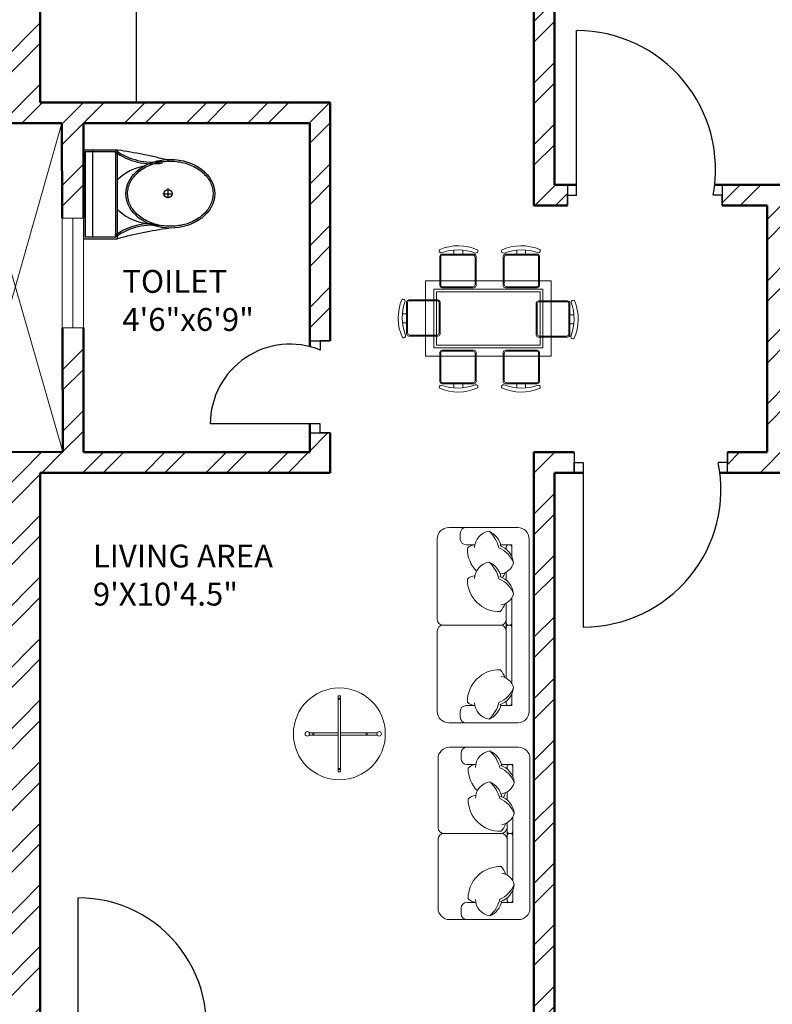
# Model space of a CAD drawing. Units: inches. Extents: x 1980 to 2738, y 1471 to 2568.
# Tile 20 of 22: x 2363 to 2528, y 2112 to 2328. Entities that reach past the tile are written whole.
import ezdxf

# ---------------------------------------------------------------- set-up
doc = ezdxf.new("R2010")
doc.units = ezdxf.units.IN
for name, color, linetype, lineweight in [('A-ANNO-DIMS', 2, 'Continuous', 18), ('A-AREA-IDEN', 7, 'Continuous', 18), ('A-DOOR', 31, 'Continuous', 25), ('A-FLOR-CASE', 8, 'Continuous', 25), ('A-FLOR-FIXT', 8, 'Continuous', 25), ('A-FLOR-OPEN', 8, 'Continuous', 18), ('A-FURN', 8, 'Continuous', 18), ('A-GLAZ', 141, 'Continuous', 18), ('A-WALL', 7, 'Continuous', 50)]:
    doc.layers.add(name, color=color, linetype=linetype, lineweight=lineweight)
doc.layers.add('A-WALL-PATT', color=9, linetype='Continuous', lineweight=13, true_color=0xd19cc7)
doc.styles.get("Standard").update_dxf_attribs({"font": 'arial.ttf'})
doc.dimstyles.get("Standard").update_dxf_attribs({"dimtxt": 0.18, "dimasz": 0.18, "dimexe": 0.18, "dimexo": 0.0625, "dimgap": 0.09, "dimtad": 0, "dimtih": 1, "dimtoh": 1, "dimdec": 4, "dimzin": 0, "dimdsep": 46, "dimtxsty": 'Standard', "dimcen": 0.09, "dimadec": 0, "dimazin": 0, "dimtfac": 1, "dimtdec": 4, "dimtofl": 0, "dimtmove": 0, "dimatfit": 3, "dimfxl": 1, "dimtolj": 1, "dimtzin": 0, "dimarcsym": 0})

# ---------------------------------------------------------------- blocks, each defined once
blk = doc.blocks.new('A$C31115884')
for p, q in [((257.5, 466.4), (257.5, 523.2)), ((283.1, 497.7), (223.4, 497.7)), ((0, 200), (0, 0)), ((520, 200), (0, 200)), ((10, 190), (10, 10)), ((510, 190), (10, 190)), ((510, 10), (510, 190)), ((520, 0), (520, 200)), ((510, 54.5), (0, 54.5)), ((10, 10), (510, 10)), ((0, 0), (520, 0))]:
    blk.add_line(p, q)
blk.add_circle((255.6, 496.4), 23.6)
for centre, radius, start, end in [((2777.7, -204.6), 2807, 165.4549, 171.71327), ((-294.5, 403.3), 364.7, 324.20913, 9.34987), ((-294.5, 403.3), 374.7, 324.20913, 9.34987), ((805.8, 403.3), 364.7, 170.65013, 215.79087), ((3237, 905), 2807, 188.28673, 194.5451), ((139.5, 406.2), 293.5, 315.84364, 2.65635), ((805.8, 403.3), 374.7, 179.20365, 215.79087), ((383.6, 406.2), 293.5, 190.27735, 224.15636)]:
    blk.add_arc(centre, radius, start, end)
blk.add_ellipse((256.2, 509.9), major_axis=(0, -260.7), ratio=0.772727)
blk.add_open_spline([(256.2, 259.2), (263.1, 259.2), (270, 259.7), (287.8, 262.3), (298.7, 265.1), (319.9, 273.1), (330.2, 278.4), (350.1, 291.1), (359.7, 298.7), (377.7, 315.9), (386.2, 325.5), (401.7, 346.6), (408.8, 358.1), (421.3, 382.5), (426.8, 395.5), (435.9, 422.4), (439.5, 436.4), (444.8, 465.1), (446.5, 479.7), (447.9, 509.2), (447.6, 524), (445, 553.3), (442.7, 567.8), (436.3, 596), (432.1, 609.7), (421.9, 636), (416, 648.6), (402.5, 672.1), (395, 683), (378.6, 703), (369.8, 712.1), (351.1, 728), (341.3, 734.8), (320.9, 746.2), (310.4, 750.7), (288.9, 757.3), (278, 759.4), (256, 761), (245, 760.6), (223.1, 757.2), (212.3, 754.3), (191.1, 746.1), (180.8, 740.7), (160.9, 727.8), (151.4, 720.1), (133.5, 702.7), (125.1, 693), (109.6, 671.7), (102.6, 660.2), (90.2, 635.7), (84.9, 622.7), (76, 595.6), (72.4, 581.6), (67.2, 552.9), (65.6, 538.2), (64.4, 508.8), (64.8, 494), (67.5, 464.7), (69.9, 450.2), (76.6, 422), (80.8, 408.3), (91.1, 382.2), (97.2, 369.7), (110.8, 346.3), (118.4, 335.4), (134.8, 315.6), (143.7, 306.7), (162.4, 290.9), (172.3, 284.2), (192.8, 273), (203.3, 268.6), (224.8, 262.2), (235.8, 260.2), (249.9, 259.3), (253, 259.2), (256.2, 259.2)], degree=3, knots=[0, 0, 0, 0, 0.110105, 0.110105, 0.285049, 0.285049, 0.459994, 0.459994, 0.634938, 0.634938, 0.809882, 0.809882, 0.984827, 0.984827, 1.159771, 1.159771, 1.334715, 1.334715, 1.50966, 1.50966, 1.684604, 1.684604, 1.859549, 1.859549, 2.034493, 2.034493, 2.209437, 2.209437, 2.384382, 2.384382, 2.559326, 2.559326, 2.73427, 2.73427, 2.909215, 2.909215, 3.084159, 3.084159, 3.259103, 3.259103, 3.434048, 3.434048, 3.608992, 3.608992, 3.783936, 3.783936, 3.958881, 3.958881, 4.133825, 4.133825, 4.30877, 4.30877, 4.483714, 4.483714, 4.658658, 4.658658, 4.833603, 4.833603, 5.008547, 5.008547, 5.183491, 5.183491, 5.358436, 5.358436, 5.53338, 5.53338, 5.708324, 5.708324, 5.883269, 5.883269, 6.058213, 6.058213, 6.233158, 6.233158, 6.283185, 6.283185, 6.283185, 6.283185])
blk = doc.blocks.new('table r 343')
at = {"color": 0}
for p, q in [((-10, 10), (-10, 262.1)), ((10, 10), (10, 262.1)), ((-330.3, 10), (330.3, 10)), ((-330.3, 10), (-330.3, -10)), ((330.3, 10), (330.3, -10)), ((-330.3, -10), (330.3, -10)), ((-10, -330.3), (-10, -10)), ((10, -330.3), (10, -10))]:
    blk.add_line(p, q, dxfattribs=at)
for centre, radius in [((0, 0), 400), ((0, 278.7), 19.4), ((0, 226.8), 5), ((-306.1, 0), 5), ((306.1, 0), 5), ((0, -238.1), 5), ((0, -346.9), 19.4)]:
    blk.add_circle(centre, radius, dxfattribs=at)
blk = doc.blocks.new('TABLE-DINING-RECT')
for points in [[(0, 16.47), (27.45, 16.47), (27.45, 0), (0, 0)], [(0, 16.47), (27.45, 16.47), (27.45, 0), (0, 0)], [(1.83, 14.64), (25.62, 14.64), (25.62, 1.83), (1.83, 1.83)], [(1.83, 14.64), (25.62, 14.64), (25.62, 1.83), (1.83, 1.83)], [(2.38, 14.09), (25.07, 14.09), (25.07, 2.38), (2.38, 2.38)], [(2.38, 14.09), (25.07, 14.09), (25.07, 2.38), (2.38, 2.38)]]:
    blk.add_lwpolyline(points, close=True)
blk = doc.blocks.new('CHAIR-DINING')
for points in [[(0.45, 7.65, -0.175809), (7.92, 7.6, 0.578392), (8.49, 8.22, 0.214524), (0.05, 8.33, 0.552014), (0.45, 7.65, -0.065079)], [(0.45, 7.65, -0.175809), (7.92, 7.6, 0.578392), (8.49, 8.22, 0.214524), (0.05, 8.33, 0.552014), (0.45, 7.65, -0.065079)], [(7.61, 7.35), (0.67, 7.35, 0.414214), (0.18, 6.87), (0.18, 0.49, 0.414214), (0.67, 0), (7.61, 0, 0.414214), (8.09, 0.49), (8.09, 6.87, 0.414214), (7.61, 7.35)], [(7.61, 7.35), (0.67, 7.35, 0.414214), (0.18, 6.87), (0.18, 0.49, 0.414214), (0.67, 0), (7.61, 0, 0.414214), (8.09, 0.49), (8.09, 6.87, 0.414214), (7.61, 7.35)], [(5.17, 7.35), (5.17, 8.23, -0.064759)], [(5.17, 7.35), (5.17, 8.23, -0.064759)]]:
    blk.add_lwpolyline(points, format="xyb")
blk.add_lwpolyline([(0.67, 7.13), (7.39, 7.13, -0.414214), (7.87, 6.65), (7.87, 0.7, -0.414214), (7.39, 0.22), (0.67, 0.22, -0.512069), (0.4, 0.7), (0.4, 6.65, -0.512069)], format="xyb", close=True)
blk.add_lwpolyline([(0.67, 7.13), (7.39, 7.13, -0.414214), (7.87, 6.65), (7.87, 0.7, -0.414214), (7.39, 0.22), (0.67, 0.22, -0.512069), (0.4, 0.7), (0.4, 6.65, -0.512069)], format="xyb", close=True)
blk.add_lwpolyline([(3.23, 8.25), (3.23, 7.35)])
blk.add_lwpolyline([(3.23, 8.25), (3.23, 7.35)])
blk = doc.blocks.new('SHAFT-OPENING-MARK')
for p, q in [((20.51, 72), (0, 0)), ((0, 72), (20.71, 0.06))]:
    blk.add_line(p, q)
blk = doc.blocks.new('*D35')
at = {"layer": 'A-ANNO-DIMS', "color": 0, "lineweight": -2, "transparency": 16777216}
for p, q in [((2081.08, 2291.77), (2081.08, 2507.54)), ((2081.26, 2507.36), (2362.79, 2507.36)), ((2644.9, 2507.36), (2363.37, 2507.36)), ((2645.08, 2291.77), (2645.08, 2507.54))]:
    blk.add_line(p, q, dxfattribs=at)
at = {"layer": 'A-ANNO-DIMS', "color": 0, "transparency": 16777216}
for points in [[(2081.26, 2507.39), (2081.26, 2507.33), (2081.08, 2507.36)], [(2644.9, 2507.39), (2644.9, 2507.33), (2645.08, 2507.36)]]:
    blk.add_solid(points, dxfattribs=at)
at = {"layer": 'Defpoints', "color": 0, "transparency": 16777216}
for p in [(2645.08, 2507.36), (2081.08, 2291.71), (2645.08, 2291.71)]:
    blk.add_point(p, dxfattribs=at)
at = {"layer": 'A-ANNO-DIMS', "color": 0, "transparency": 16777216, "insert": (2363.08, 2507.36), "char_height": 0.18, "attachment_point": 5}
blk.add_mtext('\\A1;564', dxfattribs=at)

msp = doc.modelspace()

# ---------------------------------------------------------------- hatches: boundary and pattern name
at = {"layer": 'A-WALL-PATT'}
h = msp.add_hatch(dxfattribs=at)
h.set_pattern_fill('ANSI32', color=256)
h.paths.add_polyline_path([(2257.5661, 2416.2064), (2257.5661, 2420.7064), (2250.5833, 2420.7064), (2250.5833, 2462.7064), (2246.0833, 2462.7064), (2246.0833, 2420.7064), (2237.0791, 2420.7064), (2237.0791, 2411.7064), (2246.0833, 2411.7064), (2246.0833, 2291.7064), (2242.6109, 2291.7064), (2242.6109, 2287.2064), (2246.0833, 2287.2064), (2250.5833, 2287.2064), (2250.5833, 2291.7064), (2250.5833, 2411.7064), (2257.5661, 2411.7064)])
h.paths.add_polyline_path([(2387.0396, 2416.2064), (2387.0396, 2420.7064), (2367.5833, 2420.7064), (2367.5833, 2462.7064), (2358.5833, 2462.7064), (2358.5833, 2420.7064), (2329.3087, 2420.7064), (2329.3087, 2411.7064), (2358.5833, 2411.7064), (2358.5833, 2321.7275), (2358.5833, 2309.7064), (2347.3089, 2309.7064), (2293.3089, 2309.7064), (2293.3089, 2259.0771), (2297.8089, 2259.0771), (2297.8089, 2305.2064), (2347.3089, 2305.2064), (2347.3089, 2284.7412), (2351.8089, 2284.7412), (2351.8089, 2305.2064), (2372.3188, 2305.2064), (2372.3761, 2284.3899), (2377.0295, 2284.3899), (2377.0295, 2299.3058), (2377.0295, 2305.2064), (2426.5295, 2305.2064), (2426.5295, 2257.5573), (2431.0295, 2257.5573), (2431.0295, 2309.7064), (2377.0295, 2309.7064), (2367.5833, 2309.7064), (2367.5833, 2321.7275), (2367.5833, 2411.7064), (2387.0396, 2411.7064)])
h.paths.add_polyline_path([(2448.5267, 2416.2064), (2448.5267, 2420.7064), (2423.0396, 2420.7064), (2423.0396, 2411.7064), (2448.5267, 2411.7064)])
h.paths.add_polyline_path([(2130.9128, 2416.2064), (2130.9128, 2420.7064), (2105.0833, 2420.7064), (2105.0833, 2386.6942), (2114.0833, 2386.6942), (2114.0833, 2411.7064), (2130.9128, 2411.7064)])
h.paths.add_polyline_path([(2212.9478, 2420.7064), (2190.9128, 2420.7064), (2190.9128, 2411.7064), (2212.9478, 2411.7064), (2212.9478, 2416.2064)])
h.paths.add_polyline_path([(2114.0833, 2326.6942), (2105.0833, 2326.6942), (2105.0833, 2291.7064), (2081.0833, 2291.7064), (2081.0833, 2287.2064), (2105.0833, 2287.2064), (2105.0833, 2276.1935), (2114.0833, 2276.1935), (2114.0833, 2287.2064), (2166.3825, 2287.2064), (2166.3825, 2289.4564), (2166.3825, 2291.7064), (2114.0833, 2291.7064)])
h.paths.add_polyline_path([(2114.0833, 2252.1935), (2105.0833, 2252.1935), (2105.0833, 2233.2064), (2081.0833, 2233.2064), (2081.0833, 2228.7064), (2105.0833, 2228.7064), (2105.0833, 2213.4478), (2114.0833, 2213.4478), (2114.0833, 2228.7064), (2195.0833, 2228.7064), (2199.5833, 2228.7064), (2208.4455, 2228.7064), (2208.4455, 2230.9564), (2208.4455, 2233.2064), (2199.5833, 2233.2064), (2199.5833, 2287.2064), (2206.8904, 2287.2064), (2206.8904, 2289.4564), (2206.8904, 2291.7064), (2189.446, 2291.7064), (2189.446, 2289.4564), (2189.446, 2287.2064), (2195.0833, 2287.2064), (2195.0833, 2233.2064), (2114.0833, 2233.2064)])
h.paths.add_polyline_path([(2114.0833, 2153.4478), (2109.5833, 2153.4478), (2105.0833, 2153.4478), (2105.0833, 2135.2374), (2114.0833, 2135.2374)], flags=17)
h.paths.add_polyline_path([(2135.9619, 2095.4081), (2140.1805, 2095.4081), (2140.1805, 2104.2064), (2114.0833, 2104.2064), (2114.0833, 2110.3997), (2109.5833, 2110.3997), (2105.0833, 2110.3997), (2105.0833, 2104.2064), (2081.0833, 2104.2064), (2081.0833, 2099.7064), (2105.0833, 2099.7064), (2127.5416, 2099.8532), (2127.5416, 2056.9393), (2136.2133, 2056.9393)], flags=17)
h.paths.add_polyline_path([(2255.4895, 2104.2064), (2250.5833, 2104.2064), (2250.5833, 2233.2064), (2246.0833, 2233.2064), (2242.4941, 2233.2064), (2242.4941, 2228.7064), (2246.0833, 2228.7064), (2246.0833, 2104.2064), (2163.6825, 2104.2064), (2163.6825, 2099.8072), (2163.6825, 2095.4081), (2191.4325, 2095.4081), (2191.4325, 2011.2064), (2186.0833, 2011.2064), (2136.5143, 2010.8824), (2136.3702, 2032.9403), (2131.9559, 2032.9115), (2127.5416, 2032.8826), (2127.5416, 2006.7064), (2105.0833, 2006.7064), (2081.0833, 2006.7064), (2081.0833, 2002.2064), (2105.0833, 2002.2064), (2105.0833, 1995.9329), (2114.0833, 1995.9329), (2114.0833, 2002.2064), (2246.0833, 2002.2064), (2246.0833, 1877.7064), (2242.1358, 1877.7064), (2242.1358, 1873.2064), (2250.5833, 1873.2064), (2250.5833, 2002.2064), (2255.3335, 2002.2064), (2255.3335, 2011.2064), (2195.9325, 2011.2064), (2195.9325, 2095.2064), (2255.4895, 2095.2064), (2255.4895, 2099.5471)])
h.paths.add_polyline_path([(2199.5833, 1873.2064), (2209.827, 1873.2064), (2209.827, 1875.4564), (2209.827, 1877.7064), (2114.0833, 1877.7064), (2114.0833, 1890.0968), (2105.0833, 1890.0968), (2105.0833, 1877.7064), (2081.0833, 1877.7064), (2081.0833, 1873.2064), (2105.0833, 1873.2064), (2105.0833, 1857.7279), (2114.0833, 1857.7279), (2114.0833, 1873.2064), (2195.0833, 1873.2064), (2195.0833, 1819.2064), (2190.298, 1819.2064), (2190.298, 1814.7064), (2209.8976, 1814.7064), (2209.8976, 1816.9564), (2209.8976, 1819.2064), (2199.5833, 1819.2064)])
h.paths.add_polyline_path([(2114.0833, 1814.7064), (2166.2538, 1814.7064), (2166.2538, 1816.9564), (2166.2538, 1819.2064), (2114.0833, 1819.2064), (2114.0833, 1833.7279), (2109.5833, 1833.7279), (2105.0833, 1833.7279), (2105.0833, 1819.2064), (2081.0833, 1819.2064), (2081.0833, 1814.7064), (2105.0833, 1814.7064), (2105.0833, 1782.5516), (2114.0833, 1782.5516)])
h.paths.add_polyline_path([(2114.0833, 1722.5516), (2109.5833, 1722.5516), (2105.0833, 1722.5516), (2105.0833, 1685.7064), (2124.5104, 1685.7064), (2124.5104, 1690.2064), (2124.5104, 1694.7064), (2114.0833, 1694.7064)])
h.paths.add_polyline_path([(2218.8787, 1694.7064), (2184.5104, 1694.7064), (2184.5104, 1685.7064), (2218.8787, 1685.7064), (2218.8787, 1690.2064)])
h.paths.add_polyline_path([(2250.5833, 1819.2064), (2242.6431, 1819.2064), (2242.6431, 1816.9564), (2242.6431, 1814.7064), (2246.0833, 1814.7064), (2246.0833, 1694.7064), (2240.4035, 1694.7064), (2240.4035, 1690.2064), (2240.4035, 1685.7064), (2246.0833, 1685.7064), (2246.0833, 1643.7064), (2250.5833, 1643.7064), (2250.5833, 1685.7064), (2255.9859, 1685.7064), (2255.9859, 1690.2064), (2255.9859, 1694.7064), (2250.5833, 1694.7064)])
h.paths.add_polyline_path([(2297.4764, 1694.7064), (2279.3934, 1694.7064), (2279.3934, 1690.2064), (2279.3934, 1685.7064), (2297.4764, 1685.7064), (2297.4764, 1690.2064)])
h.paths.add_polyline_path([(2377.1596, 1694.7064), (2367.5833, 1694.7064), (2367.5833, 1787.7064), (2431.0295, 1787.7064), (2431.0295, 1792.2064), (2431.0295, 1849.4149), (2428.7795, 1849.4149), (2426.5295, 1849.4149), (2426.5295, 1792.2064), (2421.5833, 1792.2064), (2367.5833, 1792.2064), (2297.8089, 1792.2064), (2297.8089, 1850.2946), (2295.5589, 1850.2946), (2293.3089, 1850.2946), (2293.3089, 1792.2064), (2293.3089, 1787.7064), (2297.8089, 1787.7064), (2358.5833, 1787.7064), (2358.5833, 1694.7064), (2333.4764, 1694.7064), (2333.4764, 1685.7064), (2358.5833, 1685.7064), (2358.5833, 1643.7064), (2367.5833, 1643.7064), (2367.5833, 1685.7064), (2377.1596, 1685.7064)])
h.paths.add_polyline_path([(2442.4912, 1694.7064), (2413.1596, 1694.7064), (2413.1596, 1685.7064), (2442.4912, 1685.7064)])
h.paths.add_polyline_path([(2480.0833, 1814.7064), (2483.4816, 1814.7064), (2483.4816, 1817.9384), (2483.4816, 1819.2064), (2475.5833, 1819.2064), (2475.5833, 1694.7064), (2470.7283, 1694.7064), (2470.7283, 1685.7064), (2475.5833, 1685.7064), (2475.5833, 1643.7064), (2480.0833, 1643.7064), (2480.0833, 1685.7064), (2486.3293, 1685.7064), (2486.3293, 1690.2064), (2486.3293, 1694.7064), (2480.0833, 1694.7064)])
h.paths.add_polyline_path([(2621.0833, 1721.7349), (2612.0833, 1721.7349), (2612.0833, 1694.7064), (2586.1453, 1694.7064), (2586.1453, 1685.7064), (2621.0833, 1685.7064)])
h.paths.add_polyline_path([(2526.1453, 1690.2064), (2526.1453, 1694.7064), (2511.584, 1694.7064), (2511.584, 1690.2064), (2511.584, 1685.7064), (2526.1453, 1685.7064)])
h.paths.add_polyline_path([(2645.0833, 1819.2064), (2621.0833, 1819.2064), (2621.0833, 1835.8527), (2616.5833, 1835.8527), (2612.0833, 1835.8527), (2612.0833, 1819.2064), (2560.2541, 1819.2064), (2560.2541, 1814.7064), (2612.0833, 1814.7064), (2612.0833, 1781.7349), (2621.0833, 1781.7349), (2621.0833, 1814.7064), (2645.0833, 1814.7064)])
h.paths.add_polyline_path([(2645.0833, 1877.7064), (2621.0833, 1877.7064), (2621.0833, 1886.4375), (2612.0833, 1886.4375), (2612.0833, 1877.7064), (2517.1032, 1877.7064), (2517.1032, 1875.4564), (2517.1032, 1873.2064), (2526.5833, 1873.2064), (2526.5833, 1819.2064), (2516.6454, 1819.2064), (2516.6454, 1816.9564), (2516.6454, 1814.7064), (2536.4445, 1814.7064), (2536.4445, 1816.9564), (2536.4445, 1819.2064), (2531.0833, 1819.2064), (2531.0833, 1873.2064), (2612.0833, 1873.2064), (2612.0833, 1859.8527), (2621.0833, 1859.8527), (2621.0833, 1873.2064), (2645.0833, 1873.2064)])
h.paths.add_polyline_path([(2645.0833, 2006.7064), (2621.0833, 2006.7064), (2588.5085, 2006.7064), (2588.5085, 2052.9125), (2579.9045, 2052.9125), (2579.9045, 2011.2064), (2519.9045, 2011.2064), (2519.9045, 2095.2064), (2553.1204, 2095.2064), (2553.1204, 2104.2064), (2480.0833, 2104.2064), (2480.0833, 2228.7064), (2484.3832, 2228.7064), (2484.3832, 2230.9564), (2484.3832, 2233.2064), (2475.5833, 2233.2064), (2475.5833, 2104.2064), (2463.1308, 2104.2064), (2463.1308, 2095.2064), (2501.2463, 2095.2064), (2510.9045, 2095.2064), (2515.4045, 2095.2064), (2515.4045, 2011.2064), (2510.9045, 2011.2064), (2501.2463, 2011.2064), (2462.5957, 2011.2064), (2462.5957, 2002.2064), (2475.5833, 2002.2064), (2475.5833, 1873.2064), (2483.6146, 1873.2064), (2483.6146, 1875.4564), (2483.6146, 1877.7064), (2480.0833, 1877.7064), (2480.0833, 2002.2064), (2612.0833, 2002.2064), (2612.0833, 1996.309), (2621.0833, 1996.309), (2621.0833, 2002.2064), (2645.0833, 2002.2064)])
h.paths.add_polyline_path([(2588.5085, 2099.7277), (2621.0833, 2099.7277), (2645.0833, 2099.7064), (2645.0833, 2104.2064), (2621.0833, 2104.2064), (2621.0833, 2109.0038), (2616.5833, 2109.0038), (2612.0833, 2109.0038), (2612.0833, 2104.2064), (2575.0621, 2104.2064), (2575.0621, 2099.7064), (2575.0621, 2095.2064), (2579.9045, 2095.2064), (2579.9045, 2076.9125), (2588.5085, 2076.9125)], flags=17)
h.paths.add_polyline_path([(2367.5833, 2002.2064), (2373.7228, 2002.2064), (2373.7228, 2006.7064), (2373.7228, 2011.2064), (2350.7889, 2011.2064), (2350.7889, 2006.7064), (2350.7889, 2002.2064), (2358.5833, 2002.2064), (2358.5833, 1877.7064), (2293.3089, 1877.7064), (2293.3089, 1870.4987), (2297.8089, 1870.4987), (2297.8089, 1873.2064), (2347.3089, 1873.2064), (2347.3089, 1847.2208), (2351.8089, 1847.2208), (2351.8089, 1873.2064), (2372.5295, 1873.2064), (2372.5295, 1847.8619), (2377.0295, 1847.8619), (2377.0295, 1873.2064), (2426.5295, 1873.2064), (2426.5295, 1868.7339), (2431.0295, 1868.7339), (2431.0295, 1877.7064), (2367.5833, 1877.7064)])
h.paths.add_polyline_path([(2531.0833, 2287.2064), (2534.2285, 2287.2064), (2534.2285, 2291.7064), (2516.7886, 2291.7064), (2516.7886, 2287.2064), (2526.5833, 2287.2064), (2526.5833, 2233.2064), (2517.9112, 2233.2064), (2517.9112, 2230.9564), (2517.9112, 2228.7064), (2526.5833, 2228.7064), (2531.0833, 2228.7064), (2612.0833, 2228.7064), (2612.0833, 2206.8504), (2621.0833, 2206.8504), (2621.0833, 2228.7064), (2645.0833, 2228.7064), (2645.0833, 2233.2064), (2621.0833, 2233.2064), (2621.0833, 2241.8536), (2616.5833, 2241.8536), (2612.0833, 2241.8536), (2612.0833, 2233.2064), (2531.0833, 2233.2064)])
h.paths.add_polyline_path([(2645.0833, 2291.7064), (2621.0833, 2291.7064), (2621.0833, 2323.0138), (2616.5833, 2323.0138), (2612.0833, 2323.0138), (2612.0833, 2291.7064), (2559.6852, 2291.7064), (2559.6852, 2289.4564), (2559.6852, 2287.2064), (2612.0833, 2287.2064), (2612.0833, 2265.8536), (2621.0833, 2265.8536), (2621.0833, 2287.2064), (2645.0833, 2287.2064)])
h.paths.add_polyline_path([(2621.0833, 2420.7064), (2582.8189, 2420.7064), (2582.8189, 2411.7064), (2612.0833, 2411.7064), (2612.0833, 2383.0138), (2621.0833, 2383.0138)])
h.paths.add_polyline_path([(2480.0833, 2411.7064), (2485.7342, 2411.7064), (2485.7342, 2416.2064), (2485.7342, 2420.7064), (2480.0833, 2420.7064), (2480.0833, 2462.7064), (2475.5833, 2462.7064), (2475.5833, 2420.7064), (2469.4083, 2420.7064), (2469.4083, 2411.7064), (2475.5833, 2411.7064), (2475.5833, 2291.7064), (2475.5833, 2287.2064), (2482.9195, 2287.2064), (2482.9195, 2289.4564), (2482.9195, 2291.7064), (2480.0833, 2291.7064)])
h.paths.add_polyline_path([(2367.5833, 2228.7064), (2431.0295, 2228.7064), (2431.0295, 2233.2064), (2431.0295, 2237.4203), (2428.7795, 2237.4203), (2426.5295, 2237.4203), (2426.5295, 2233.2064), (2377.0295, 2233.2064), (2377.0295, 2260.3837), (2372.4423, 2260.3837), (2372.517, 2233.2635), (2351.8089, 2233.2064), (2351.8089, 2260.7412), (2347.3089, 2260.7412), (2347.3089, 2233.2064), (2297.8089, 2233.2064), (2297.8089, 2236.9324), (2293.3089, 2236.9324), (2293.3089, 2228.7064), (2358.5833, 2228.7064), (2358.5833, 2104.2064), (2353.3665, 2104.2064), (2353.3665, 2095.2064), (2373.8869, 2095.2064), (2373.8869, 2099.7064), (2373.8869, 2104.2064), (2367.5833, 2104.2064)])
h.paths.add_polyline_path([(2321.2323, 2104.2064), (2303.4895, 2104.2064), (2303.4895, 2095.2064), (2321.2323, 2095.2064), (2321.2323, 2099.7064)], flags=0)
h.paths.add_polyline_path([(2415.1308, 2099.7064), (2415.1308, 2104.2064), (2404.81, 2104.2064), (2404.81, 2095.2064), (2415.1308, 2095.2064)], flags=17)
h.paths.add_polyline_path([(2318.6336, 2011.2064), (2303.3335, 2011.2064), (2303.3335, 2002.2064), (2318.6336, 2002.2064)], flags=0)
h.paths.add_polyline_path([(2414.5957, 2011.2064), (2406.2461, 2011.2064), (2406.2461, 2006.7064), (2406.2461, 2002.2064), (2414.5957, 2002.2064)], flags=17)

# ---------------------------------------------------------------- linework, layer by layer
at = {"layer": 'A-DOOR'}
for p, q in [((2484.9195, 2289.4564), (2484.9195, 2325.4564)), ((2482.9195, 2291.7064), (2482.9195, 2291.7064)), ((2482.9195, 2291.7064), (2482.9195, 2287.2064)), ((2516.7886, 2291.7064), (2516.7886, 2287.2064)), ((2482.9195, 2287.2064), (2482.9195, 2289.4564)), ((2482.9195, 2289.4564), (2484.9195, 2289.4564)), ((2516.7886, 2289.4564), (2514.7886, 2289.4564)), ((2516.7886, 2287.2064), (2516.7886, 2289.4564)), ((2426.5295, 2257.5573), (2431.0295, 2257.5573)), ((2431.0295, 2257.5573), (2428.7795, 2257.5573)), ((2428.7795, 2257.5573), (2428.7795, 2255.5573)), ((2428.7795, 2239.4203), (2404.7795, 2239.4203)), ((2428.7795, 2237.4203), (2428.7795, 2239.4203)), ((2426.5295, 2237.4203), (2431.0295, 2237.4203)), ((2431.0295, 2237.4203), (2428.7795, 2237.4203)), ((2484.3832, 2233.2064), (2484.3832, 2228.7064)), ((2517.9112, 2228.7064), (2517.9112, 2233.2064)), ((2517.9112, 2233.2064), (2517.9112, 2230.9564)), ((2484.3832, 2228.7064), (2484.3832, 2230.9564)), ((2484.3832, 2230.9564), (2486.3832, 2230.9564)), ((2486.3832, 2230.9564), (2486.3832, 2194.9564)), ((2517.9112, 2230.9564), (2515.9112, 2230.9564)), ((2375.8869, 2099.7064), (2375.8869, 2135.7064))]:
    msp.add_line(p, q, dxfattribs=at)
for centre, radius, start, end in [((2484.9195, 2295.0653), 30.3911, 349.364739, 90), ((2422.2046, 2239.4203), 17.4251, 67.831899, 180), ((2486.3832, 2225.0661), 30.1097, 270, 11.281357), ((2375.8869, 2107.639), 28.0674, 343.583066, 90)]:
    msp.add_arc(centre, radius, start, end, dxfattribs=at)
at = {"layer": 'A-FLOR-CASE'}
msp.add_line((2388.6126, 2309.7064), (2388.6126, 2397.4159), dxfattribs=at)
at = {"layer": 'A-FURN'}
for points in [[(2469.0499, 2276.7849, -0.57839206), (2468.4835, 2277.4076, -0.21452438), (2476.9217, 2277.5209, -0.55201397), (2476.5253, 2276.8415, 0.1758092), (2469.0499, 2276.7849)], [(2469.0499, 2276.7846, -0.57839206), (2468.4835, 2277.4074, -0.21452438), (2476.9217, 2277.5206, -0.55201397), (2476.5253, 2276.8413, 0.1758092), (2469.0499, 2276.7846)], [(2471.8047, 2276.5415), (2471.8047, 2277.4192, 0.06475861)], [(2471.8047, 2276.5412), (2471.8047, 2277.4189, 0.06475861)], [(2476.3069, 2276.5415, -0.41421356), (2476.7925, 2276.056), (2476.7925, 2269.6748, -0.41421356), (2476.3069, 2269.1893), (2469.367, 2269.1893, -0.41421356), (2468.8815, 2269.6748), (2468.8815, 2276.056, -0.41421356), (2469.367, 2276.5415), (2476.3069, 2276.5415)], [(2476.307, 2276.5412, -0.41421356), (2476.7925, 2276.0557), (2476.7925, 2269.6746, -0.41421356), (2476.307, 2269.189), (2469.367, 2269.189, -0.41421356), (2468.8815, 2269.6746), (2468.8815, 2276.0557, -0.41421356), (2469.367, 2276.5412), (2476.307, 2276.5412)], [(2447.4603, 2258.7895, -0.57839206), (2446.8376, 2258.2232, -0.21452438), (2446.7244, 2266.6614, -0.55201397), (2447.4037, 2266.2649, 0.17580937), (2447.4603, 2258.7895)], [(2447.4603, 2258.7892, -0.57839206), (2446.8376, 2258.2229, -0.21452438), (2446.7244, 2266.6611, -0.55201397), (2447.4037, 2266.2646, 0.17580937), (2447.4603, 2258.7892)], [(2447.7037, 2266.0466, -0.41421356), (2448.1893, 2266.5321), (2454.5704, 2266.5321, -0.41421356), (2455.0559, 2266.0466), (2455.0559, 2259.1066, -0.41421356), (2454.5704, 2258.6211), (2448.1893, 2258.6211, -0.41421356), (2447.7037, 2259.1066), (2447.7037, 2266.0466)], [(2447.7037, 2266.0463, -0.41421356), (2448.1893, 2266.5318), (2454.5704, 2266.5318, -0.41421356), (2455.0559, 2266.0463), (2455.0559, 2259.1064, -0.41421356), (2454.5704, 2258.6208), (2448.1893, 2258.6208, -0.41421356), (2447.7037, 2259.1064), (2447.7037, 2266.0463)], [(2483.7412, 2266.0273, -0.17580919), (2483.6846, 2258.5518, 0.57839206), (2484.3073, 2257.9855, 0.21452438), (2484.4206, 2266.4237, 0.55201397), (2483.7412, 2266.0273, -0.06507904)], [(2483.7412, 2266.027, -0.17580919), (2483.6846, 2258.5515, 0.57839206), (2484.3073, 2257.9852, 0.21452438), (2484.4206, 2266.4234, 0.55201397), (2483.7412, 2266.027, -0.06507904)], [(2483.4412, 2265.8089, 0.41421356), (2482.9557, 2266.2944), (2476.5745, 2266.2944, 0.41421356), (2476.089, 2265.8089), (2476.089, 2258.869, 0.41421356), (2476.5745, 2258.3834), (2482.9557, 2258.3834, 0.41421356), (2483.4412, 2258.869), (2483.4412, 2265.8089)], [(2483.4412, 2265.8086, 0.41421356), (2482.9557, 2266.2941), (2476.5745, 2266.2941, 0.41421356), (2476.089, 2265.8086), (2476.089, 2258.8687, 0.41421356), (2476.5745, 2258.3832), (2482.9557, 2258.3832, 0.41421356), (2483.4412, 2258.8687), (2483.4412, 2265.8086)], [(2447.7037, 2261.5443), (2446.826, 2261.5443, 0.06475861)], [(2447.7037, 2261.544), (2446.8261, 2261.544, 0.06475861)], [(2483.4412, 2261.3066), (2484.3189, 2261.3066, -0.06475861)], [(2483.4412, 2261.3063), (2484.3189, 2261.3063, -0.06475861)], [(2462.4393, 2248.1758), (2455.4994, 2248.1758, -0.41421356), (2455.0139, 2248.6613), (2455.0139, 2255.0424, -0.41421356), (2455.4994, 2255.528), (2462.4393, 2255.528, -0.41421356), (2462.9249, 2255.0424), (2462.9249, 2248.6613, -0.41421356), (2462.4393, 2248.1758)], [(2462.4394, 2248.1755), (2455.4994, 2248.1755, -0.41421356), (2455.0139, 2248.661), (2455.0139, 2255.0421, -0.41421356), (2455.4994, 2255.5277), (2462.4394, 2255.5277, -0.41421356), (2462.9249, 2255.0421), (2462.9249, 2248.661, -0.41421356), (2462.4394, 2248.1755)], [(2476.3069, 2248.1758, 0.41421356), (2476.7925, 2248.6613), (2476.7925, 2255.0424, 0.41421356), (2476.3069, 2255.528), (2469.367, 2255.528, 0.41421356), (2468.8815, 2255.0424), (2468.8815, 2248.6613, 0.41421356), (2469.367, 2248.1758), (2476.3069, 2248.1758)], [(2476.307, 2248.1755, 0.41421356), (2476.7925, 2248.661), (2476.7925, 2255.0421, 0.41421356), (2476.307, 2255.5277), (2469.367, 2255.5277, 0.41421356), (2468.8815, 2255.0421), (2468.8815, 2248.661, 0.41421356), (2469.367, 2248.1755), (2476.307, 2248.1755)], [(2462.7565, 2247.9323, -0.57839206), (2463.3228, 2247.3096, -0.21452438), (2454.8846, 2247.1964, -0.55201397), (2455.2811, 2247.8757, 0.17580929), (2462.7565, 2247.9323)], [(2462.7565, 2247.9321, -0.57839206), (2463.3228, 2247.3093, -0.21452438), (2454.8846, 2247.1961, -0.55201397), (2455.2811, 2247.8754, 0.17580929), (2462.7565, 2247.9321)], [(2460.0017, 2248.1758), (2460.0017, 2247.2981, 0.06475861)], [(2460.0017, 2248.1755), (2460.0017, 2247.2978, 0.06475861)], [(2476.5253, 2247.8757, -0.17580928), (2469.0499, 2247.9323, 0.57839206), (2468.4835, 2247.3096, 0.21452438), (2476.9217, 2247.1964, 0.55201397), (2476.5253, 2247.8757, -0.06507904)], [(2476.5253, 2247.8754, -0.17580928), (2469.0499, 2247.9321, 0.57839206), (2468.4835, 2247.3093, 0.21452438), (2476.9217, 2247.1961, 0.55201397), (2476.5253, 2247.8754, -0.06507904)], [(2471.8047, 2248.1758), (2471.8047, 2247.2981, -0.06475861)], [(2471.8047, 2248.1755), (2471.8047, 2247.2978, -0.06475861)], [(2462.6701, 2212.9481), (2460.7226, 2212.9481, -0.41421356), (2459.4657, 2214.205), (2459.4657, 2215.4619, -0.41421356), (2460.7226, 2216.7189)], [(2462.594, 2212.3173, -0.35677236), (2465.7622, 2215.9189, -0.24954205), (2468.3731, 2212.6555, 9.61688035)], [(2465.7622, 2215.9189, -0.14772988), (2467.9223, 2212.2453, -0.21334276), (2471.0906, 2209.0039, -0.17866181)], [(2462.6706, 2212.9508, 0.16554063), (2461.0099, 2212.1733, 0.20023115), (2463.0325, 2207.1838, 0.12152332)], [(2468.0945, 2212.7528, -0.30666349), (2471.0906, 2209.0039, -0.30632997), (2468.3544, 2206.5548, 0.87284716)], [(2470.778, 2210.3039), (2470.778, 2212.9481), (2468.3078, 2212.9481, -0.41421356)], [(2469.5211, 2211.9889), (2469.5211, 2212.4453, -0.41421356), (2470.0238, 2212.9481), (2470.2752, 2212.9481, -0.41421356), (2470.778, 2212.4453)], [(2462.594, 2205.5464, -0.35677236), (2465.7622, 2209.1479, -0.24954205), (2468.3731, 2205.8846, 9.61688035)], [(2465.7622, 2209.1479, -0.14772988), (2467.9223, 2205.4743, -0.21334276), (2471.0906, 2202.2329, -0.17866181)], [(2462.6706, 2206.1799, 0.16554063), (2461.0099, 2205.4023, 0.42598917), (2468.2104, 2198.3432, 0.12152332), (2469.2028, 2200.0189, -7.11546429)], [(2468.7114, 2205.7361, 0.07186538), (2469.2028, 2206.7899, -7.11546429)], [(2469.5211, 2205.218), (2469.5211, 2206.9472, -0.41421356)], [(2468.0945, 2205.9818, -0.30666349), (2471.0906, 2202.2329, -0.30632997), (2468.3544, 2199.7838, 0.87284716)], [(2470.778, 2201.4419), (2470.778, 2195.854, -0.41421356), (2470.2752, 2195.3513), (2470.0238, 2195.3513, -0.41421356), (2469.5211, 2195.854), (2469.5211, 2200.1762, -0.41421356)], [(2469.5211, 2196.6082, -0.41421356), (2468.2642, 2195.3513), (2455.695, 2195.3513, -0.41421356)], [(2469.5211, 2194.0943, 0.41421356), (2468.2642, 2195.3513), (2455.695, 2195.3513, 0.41421356)], [(2469.5211, 2196.6082, -0.41421356), (2468.2642, 2195.3513)], [(2469.5211, 2194.0943, 0.41421356), (2468.2642, 2195.3513)], [(2470.778, 2182.4897), (2470.778, 2194.8485, 0.41421356), (2470.2752, 2195.3513), (2470.0238, 2195.3513, 0.41421356), (2469.5211, 2194.8485), (2469.5211, 2183.7553, 0.41421356)], [(2462.6706, 2177.7517, -0.16554063), (2461.0099, 2178.5293, -0.42598917), (2468.2104, 2185.5883, -0.12152332), (2469.2028, 2183.9126, 7.11546429)], [(2468.0945, 2177.9497, 0.30666349), (2471.0906, 2181.6986, 0.30632997), (2468.3544, 2184.1477, -0.87284716)], [(2465.7622, 2174.7836, 0.14772988), (2467.9223, 2178.4572, 0.21334276), (2471.0906, 2181.6986, 0.17866181)], [(2462.594, 2178.3852, 0.35677236), (2465.7622, 2174.7836, 0.24954205), (2468.3731, 2178.047, -9.61688035)], [(2469.5211, 2178.7136), (2469.5211, 2178.2572, 0.41421356), (2470.0238, 2177.7544), (2470.2752, 2177.7544, 0.41421356), (2470.778, 2178.2572)], [(2460.7226, 2173.9837, -0.41421356), (2459.4657, 2175.2406), (2459.4657, 2176.4975, -0.41421356), (2460.7226, 2177.7544), (2462.6701, 2177.7544)], [(2462.8389, 2164.8704), (2460.8915, 2164.8704, -0.41421356), (2459.6346, 2166.1273), (2459.6346, 2167.3842, -0.41421356), (2460.8915, 2168.6411)], [(2462.7629, 2164.2396, -0.35677236), (2465.9311, 2167.8412, -0.24954205), (2468.5419, 2164.5778, 9.61688035)], [(2465.9311, 2167.8412, -0.14772988), (2468.0912, 2164.1676, -0.21334276), (2471.2594, 2160.9261, -0.17866181)], [(2462.8395, 2164.8731, 0.16554063), (2461.1788, 2164.0955, 0.20023115), (2463.2014, 2159.106, 0.12152332)], [(2468.2634, 2164.6751, -0.30666349), (2471.2594, 2160.9261, -0.30632997), (2468.5232, 2158.4771, 0.87284716)], [(2470.9468, 2162.2262), (2470.9468, 2164.8704), (2468.4767, 2164.8704, -0.41421356)], [(2469.6899, 2163.9112), (2469.6899, 2164.3676, -0.41421356), (2470.1927, 2164.8704), (2470.4441, 2164.8704, -0.41421356), (2470.9468, 2164.3676)], [(2462.7629, 2157.4686, -0.35677236), (2465.9311, 2161.0702, -0.24954205), (2468.5419, 2157.8069, 9.61688035)], [(2465.9311, 2161.0702, -0.14772988), (2468.0912, 2157.3966, -0.21334276), (2471.2594, 2154.1552, -0.17866181)], [(2468.8803, 2157.6584, 0.07186538), (2469.3717, 2158.7121, -7.11546429)], [(2469.6899, 2157.1402), (2469.6899, 2158.8695, -0.41421356)], [(2462.8395, 2158.1021, 0.16554063), (2461.1788, 2157.3246, 0.42598917), (2468.3792, 2150.2655, 0.12152332), (2469.3717, 2151.9412, -7.11546429)], [(2468.2634, 2157.9041, -0.30666349), (2471.2594, 2154.1552, -0.30632997), (2468.5232, 2151.7061, 0.87284716)], [(2470.9468, 2153.3641), (2470.9468, 2150.2901, -0.41421356), (2470.4441, 2149.7874), (2470.1927, 2149.7874, -0.41421356), (2469.6899, 2150.2901), (2469.6899, 2152.0985, -0.41421356)], [(2469.6899, 2151.0443, -0.41421356), (2468.433, 2149.7874), (2455.8638, 2149.7874, -0.41421356)], [(2469.6899, 2151.0443, -0.41421356), (2468.433, 2149.7874)], [(2469.6899, 2148.5304, 0.41421356), (2468.433, 2149.7874), (2455.8638, 2149.7874, 0.41421356)], [(2469.6899, 2148.5304, 0.41421356), (2468.433, 2149.7874)], [(2470.9468, 2139.4396), (2470.9468, 2149.2846, 0.41421356), (2470.4441, 2149.7874), (2470.1927, 2149.7874, 0.41421356), (2469.6899, 2149.2846), (2469.6899, 2140.7053, 0.41421356)], [(2462.8395, 2134.7016, -0.16554063), (2461.1788, 2135.4792, -0.42598917), (2468.3792, 2142.5383, -0.12152332), (2469.3717, 2140.8626, 7.11546429)], [(2468.2634, 2134.8996, 0.30666349), (2471.2594, 2138.6486, 0.30632997), (2468.5232, 2141.0977, -0.87284716)], [(2465.9311, 2131.7336, 0.14772988), (2468.0912, 2135.4072, 0.21334276), (2471.2594, 2138.6486, 0.17866181)], [(2462.7629, 2135.3351, 0.35677236), (2465.9311, 2131.7336, 0.24954205), (2468.5419, 2134.9969, -9.61688035)], [(2469.6899, 2135.6635), (2469.6899, 2135.2071, 0.41421356), (2470.1927, 2134.7044), (2470.4441, 2134.7044, 0.41421356), (2470.9468, 2135.2071)], [(2460.8915, 2130.9336, -0.41421356), (2459.6346, 2132.1905), (2459.6346, 2133.4474, -0.41421356), (2460.8915, 2134.7044), (2462.8389, 2134.7044)]]:
    msp.add_lwpolyline(points, format="xyb", dxfattribs=at)
for points in [[(2473.7473, 2277.4352), (2473.7473, 2276.5415)], [(2473.7473, 2277.4349), (2473.7473, 2276.5412)], [(2446.8101, 2263.4869), (2447.7037, 2263.4869)], [(2446.8101, 2263.4866), (2447.7037, 2263.4866)], [(2484.3348, 2263.2492), (2483.4412, 2263.2492)], [(2484.3349, 2263.2489), (2483.4412, 2263.2489)], [(2458.0591, 2247.2821), (2458.0591, 2248.1758)], [(2458.0591, 2247.2818), (2458.0591, 2248.1755)], [(2473.7473, 2247.2821), (2473.7473, 2248.1758)], [(2473.7473, 2247.2818), (2473.7473, 2248.1755)], [(2468.3078, 2177.7544), (2470.778, 2177.7544), (2470.778, 2180.3986)], [(2468.4767, 2134.7044), (2470.9468, 2134.7044), (2470.9468, 2137.3486)]]:
    msp.add_lwpolyline(points, dxfattribs=at)
for points in [[(2476.304, 2276.3228), (2469.5857, 2276.3228, 0.41421356), (2469.1002, 2275.8373), (2469.1002, 2269.8936, 0.41421356), (2469.5857, 2269.408), (2476.304, 2269.408, 0.51206948), (2476.5737, 2269.8936), (2476.5737, 2275.8373, 0.51206948)], [(2476.304, 2276.3225), (2469.5857, 2276.3225, 0.41421356), (2469.1002, 2275.837), (2469.1002, 2269.8933, 0.41421356), (2469.5857, 2269.4078), (2476.304, 2269.4078, 0.51206948), (2476.5738, 2269.8933), (2476.5738, 2275.837, 0.51206948)], [(2447.9225, 2266.0436), (2447.9225, 2259.3254, 0.41421356), (2448.408, 2258.8399), (2454.3517, 2258.8399, 0.41421356), (2454.8372, 2259.3254), (2454.8372, 2266.0436, 0.51206948), (2454.3517, 2266.3134), (2448.408, 2266.3134, 0.51206948)], [(2447.9225, 2266.0434), (2447.9225, 2259.3251, 0.41421356), (2448.408, 2258.8396), (2454.3517, 2258.8396, 0.41421356), (2454.8372, 2259.3251), (2454.8372, 2266.0434, 0.51206948), (2454.3517, 2266.3131), (2448.408, 2266.3131, 0.51206948)], [(2483.2225, 2265.806), (2483.2225, 2259.0877, -0.41421356), (2482.7369, 2258.6022), (2476.7933, 2258.6022, -0.41421356), (2476.3077, 2259.0877), (2476.3077, 2265.806, -0.51206948), (2476.7933, 2266.0757), (2482.7369, 2266.0757, -0.51206948)], [(2483.2225, 2265.8057), (2483.2225, 2259.0874, -0.41421356), (2482.737, 2258.6019), (2476.7933, 2258.6019, -0.41421356), (2476.3077, 2259.0874), (2476.3077, 2265.8057, -0.51206948), (2476.7933, 2266.0754), (2482.737, 2266.0754, -0.51206948)], [(2455.5023, 2248.3945), (2462.2206, 2248.3945, 0.41421356), (2462.7061, 2248.88), (2462.7061, 2254.8237, 0.41421356), (2462.2206, 2255.3092), (2455.5023, 2255.3092, 0.51206948), (2455.2326, 2254.8237), (2455.2326, 2248.88, 0.51206948)], [(2455.5024, 2248.3942), (2462.2206, 2248.3942, 0.41421356), (2462.7062, 2248.8797), (2462.7062, 2254.8234, 0.41421356), (2462.2206, 2255.3089), (2455.5024, 2255.3089, 0.51206948), (2455.2326, 2254.8234), (2455.2326, 2248.8797, 0.51206948)], [(2476.304, 2248.3945), (2469.5857, 2248.3945, -0.41421356), (2469.1002, 2248.88), (2469.1002, 2254.8237, -0.41421356), (2469.5857, 2255.3092), (2476.304, 2255.3092, -0.51206948), (2476.5737, 2254.8237), (2476.5737, 2248.88, -0.51206948)], [(2476.304, 2248.3942), (2469.5857, 2248.3942, -0.41421356), (2469.1002, 2248.8797), (2469.1002, 2254.8234, -0.41421356), (2469.5857, 2255.3089), (2476.304, 2255.3089, -0.51206948), (2476.5738, 2254.8234), (2476.5738, 2248.8797, -0.51206948)], [(2470.778, 2194.8485), (2470.778, 2195.854, -0.41421356), (2470.2752, 2195.3513), (2470.0238, 2195.3513, -0.41421356), (2469.5211, 2195.854), (2469.5211, 2194.8485, -0.41421356), (2470.0238, 2195.3513), (2470.2752, 2195.3513, -0.41421356)], [(2470.9468, 2149.2846), (2470.9468, 2150.2901, -0.41421356), (2470.4441, 2149.7874), (2470.1927, 2149.7874, -0.41421356), (2469.6899, 2150.2901), (2469.6899, 2149.2846, -0.41421356), (2470.1927, 2149.7874), (2470.4441, 2149.7874, -0.41421356)]]:
    msp.add_lwpolyline(points, format="xyb", close=True, dxfattribs=at)
at = {"layer": 'A-FURN', "ltscale": 0.03}
for points in [[(2454.4381, 2194.0943, -0.41421356), (2455.695, 2195.3513, -0.41421356), (2454.4381, 2196.6082), (2454.4381, 2214.205, -0.41421356), (2456.9519, 2216.7189), (2472.0349, 2216.7189, -0.41421356), (2474.5487, 2214.205), (2474.5487, 2176.4975, -0.41421356), (2472.0349, 2173.9837), (2456.9519, 2173.9837, -0.41421356), (2454.4381, 2176.4975), (2454.4381, 2194.0943, -0.41421356), (2455.695, 2195.3513, -0.41421356), (2454.4381, 2196.6082)], [(2454.6069, 2148.5304, -0.41421356), (2455.8638, 2149.7874, -0.41421356), (2454.6069, 2151.0443), (2454.6069, 2166.1273, -0.41421356), (2457.1208, 2168.6411), (2472.2038, 2168.6411, -0.41421356), (2474.7176, 2166.1273), (2474.7176, 2133.4474, -0.41421356), (2472.2038, 2130.9336), (2457.1208, 2130.9336, -0.41421356), (2454.6069, 2133.4474), (2454.6069, 2148.5304, -0.41421356), (2455.8638, 2149.7874, -0.41421356), (2454.6069, 2151.0443)]]:
    msp.add_lwpolyline(points, format="xyb", dxfattribs=at)
at = {"layer": 'A-GLAZ'}
for p, q in [((2372.3761, 2284.3899), (2377.0295, 2284.3899)), ((2372.3761, 2284.3899), (2372.3761, 2260.3837)), ((2377.0295, 2284.3899), (2374.7028, 2284.3899)), ((2374.7028, 2284.3899), (2374.7028, 2260.3899)), ((2377.0295, 2284.3899), (2377.0295, 2260.3837)), ((2374.7028, 2260.3899), (2372.4423, 2260.3837)), ((2372.4423, 2260.3837), (2377.0295, 2260.3837))]:
    msp.add_line(p, q, dxfattribs=at)
at = {"layer": 'A-WALL'}
for p, q in [((2367.5833, 2411.7064), (2367.5833, 2321.7275)), ((2475.5833, 2411.7064), (2475.5833, 2291.7064)), ((2480.0833, 2411.7064), (2480.0833, 2291.7064)), ((2367.5833, 2309.7064), (2367.5833, 2321.7275)), ((2367.5833, 2309.7064), (2377.0295, 2309.7064)), ((2431.0295, 2309.7064), (2377.0295, 2309.7064)), ((2431.0295, 2257.5573), (2431.0295, 2309.7064)), ((2372.3188, 2305.2064), (2351.8089, 2305.2064)), ((2372.3761, 2284.3899), (2372.3188, 2305.2064)), ((2377.0295, 2305.2064), (2377.0295, 2284.3899)), ((2377.0295, 2305.2064), (2426.5295, 2305.2064)), ((2426.5295, 2305.2064), (2426.5295, 2256.3001)), ((2475.5833, 2287.2064), (2475.5833, 2291.7064)), ((2480.0833, 2291.7064), (2484.9195, 2291.7064)), ((2515.1245, 2291.7064), (2534.2285, 2291.7064)), ((2475.5833, 2287.2064), (2482.9195, 2287.2064)), ((2475.5833, 2287.2064), (2475.5833, 2287.2064)), ((2516.7886, 2287.2064), (2526.5833, 2287.2064)), ((2526.5833, 2233.2064), (2526.5833, 2287.2064)), ((2372.517, 2233.2635), (2372.4423, 2260.3837)), ((2377.0295, 2260.3837), (2377.0295, 2233.2064)), ((2426.5295, 2239.4203), (2426.5295, 2233.2064)), ((2431.0295, 2233.2064), (2431.0295, 2237.4203)), ((2351.8089, 2233.2064), (2372.517, 2233.2635)), ((2377.0295, 2233.2064), (2426.5295, 2233.2064)), ((2377.0295, 2233.2064), (2377.0295, 2233.2064)), ((2431.0295, 2233.2064), (2431.0295, 2228.7064)), ((2475.5833, 2233.2064), (2475.5833, 2104.2064)), ((2484.3832, 2233.2064), (2475.5833, 2233.2064)), ((2526.5833, 2233.2064), (2517.9112, 2233.2064)), ((2431.0295, 2228.7064), (2367.5833, 2228.7064)), ((2367.5833, 2104.2064), (2367.5833, 2228.7064)), ((2431.0295, 2228.7064), (2431.0295, 2228.7064)), ((2480.0833, 2228.7064), (2480.0833, 2104.2064)), ((2486.3832, 2228.7064), (2480.0833, 2228.7064)), ((2526.5833, 2228.7064), (2516.2721, 2228.7064)), ((2531.0833, 2228.7064), (2526.5833, 2228.7064))]:
    msp.add_line(p, q, dxfattribs=at)

# ---------------------------------------------------------------- block references
at = {"layer": 'A-FLOR-FIXT', "xscale": 0.0372717239612423, "yscale": 0.0372717239612423, "zscale": 0.0372717239612423, "rotation": 270}
msp.add_blockref('A$C31115884', (2377.0295, 2299.3058), dxfattribs=at)
at = {"layer": 'A-FLOR-OPEN'}
msp.add_blockref('SHAFT-OPENING-MARK', (2351.809, 2233.206), dxfattribs=at)
at = {"layer": 'A-FURN'}
for name, p in [('CHAIR-DINING', (2454.8321, 2269.189)), ('TABLE-DINING-RECT', (2451.8861, 2254.213))]:
    msp.add_blockref(name, p, dxfattribs=at)
at = {"layer": 'A-FURN', "xscale": 0.0251383443972704, "yscale": 0.0251383443972704, "zscale": 0.0251383443972704, "rotation": 89.99999999999999}
msp.add_blockref('table r 343', (2433.0151, 2171.5682), dxfattribs=at)

# ---------------------------------------------------------------- texts
at = {"layer": 'A-AREA-IDEN', "char_height": 5, "attachment_point": 1}
for s, width, insert in [('TOILET\\P4\'6"x6\'9"', 84.875379, (2385.5244, 2273.0784)), ('LIVING AREA\\P9\'X10\'4.5"', 117.751796, (2379.0836, 2212.9827))]:
    msp.add_mtext_dynamic_manual_height_columns(s, width=width, gutter_width=12.5, heights=[0], dxfattribs=dict(at, insert=insert))

# ---------------------------------------------------------------- dimensions: what is measured, and where the dimension line sits
at = {"layer": 'A-ANNO-DIMS'}
dim = msp.add_linear_dim(base=(2645.0833, 2507.3564), p1=(2081.0833, 2291.7064), p2=(2645.0833, 2291.7064), dimstyle='Standard', override={"dimdec": 0, "dimlfac": 1, "dimrnd": 0, "dimzin": 0, "dimdsep": 46, "dimlunit": 2}, dxfattribs=at)
dim.commit()
dim.dimension.update_dxf_attribs({"geometry": '*D35', "text_midpoint": (2363.0833, 2507.3564)})

doc.saveas('drawing.dxf')
